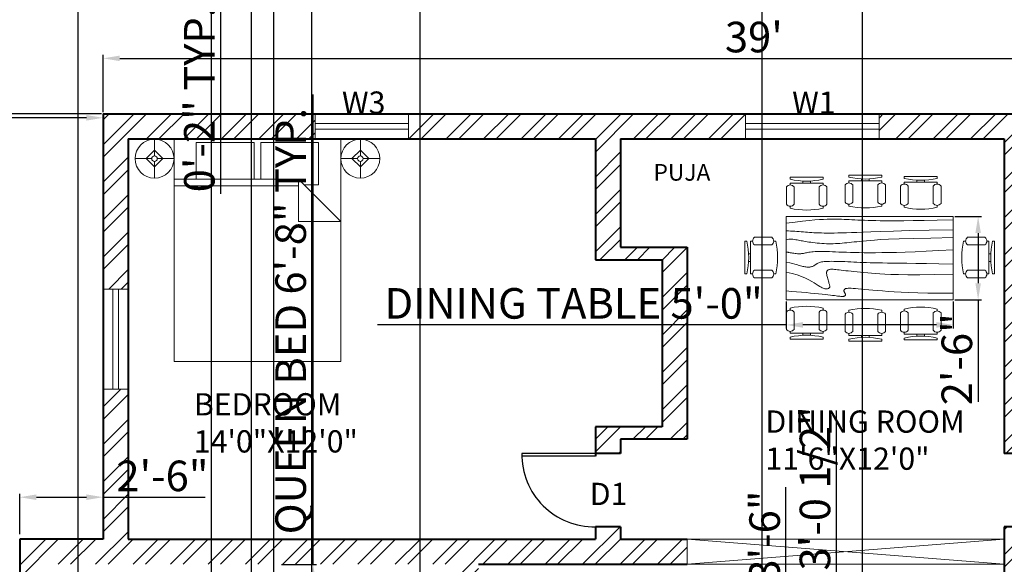
# Model space of a CAD drawing. Units: inches. Extents: x 2069 to 3028, y 691 to 1726.
# Tile 8 of 10: x 2268 to 2622, y 1325 to 1521. Entities that reach past the tile are written whole.
import ezdxf

# ---------------------------------------------------------------- set-up
doc = ezdxf.new("R2010")
doc.units = ezdxf.units.IN
for name, color, linetype, lineweight in [('A-ANNO-DIMS', 2, 'Continuous', 18), ('A-DOOR', 3, 'Continuous', 25), ('A-FURN', 8, 'Continuous', 18), ('A-GLAZ', 4, 'Continuous', 20), ('A-WALL', 7, 'Continuous', 40)]:
    doc.layers.add(name, color=color, linetype=linetype, lineweight=lineweight)
for name, color, linetype, lineweight, true_color in [('A-ANNO-TEXT', 11, 'Continuous', 18, 0xf27172), ('A-AREA-IDEN', 11, 'Continuous', 25, 0xf27172), ('A-WALL-OPEN', 143, 'Continuous', 20, 0x7aafdf), ('A-WALL-PATT', 143, 'Continuous', 13, 0x7aafdf)]:
    doc.layers.add(name, color=color, linetype=linetype, lineweight=lineweight, true_color=true_color)
doc.styles.get("Standard").update_dxf_attribs({"font": 'arial.ttf'})
doc.dimstyles.new('ISO-25', dxfattribs={"dimtxt": 11, "dimasz": 6, "dimexe": 1.25, "dimexo": 0.625, "dimtad": 1, "dimlunit": 3, "dimtxsty": 'Standard', "dimcen": 2.5, "dimclrd": 3, "dimclre": 5, "dimclrt": 6, "dimadec": 0, "dimazin": 0, "dimtfac": 1, "dimtmove": 0, "dimatfit": 3, "dimfxl": 1, "dimarcsym": 0})

# ---------------------------------------------------------------- blocks, each defined once
blk = doc.blocks.new('Table - Rectangular Woodgrain 60 x 30 in.')
for p, q in [((0, 0), (0, -30)), ((60, 0), (0, 0)), ((60, -30), (60, 0)), ((0, -30), (60, -30))]:
    blk.add_line(p, q)
for points in [[(0, -2.4), (4.8155, -2.418), (9.0302, -2.4688), (12.709, -2.5477), (15.9167, -2.65), (18.7181, -2.7711), (21.1781, -2.9063), (23.3616, -3.0508), (25.3333, -3.2), (27.1477, -3.3495), (28.8172, -3.4958), (30.3437, -3.636), (31.7291, -3.7667), (32.9756, -3.8849), (34.0849, -3.9875), (35.059, -4.0714), (35.9, -4.1334), (36.6114, -4.1711), (37.2041, -4.1854), (37.6906, -4.1779), (38.0833, -4.15), (38.3948, -4.1034), (38.6375, -4.0396), (38.8239, -3.9602), (38.9666, -3.8667), (39.0764, -3.7608), (39.1573, -3.6448), (39.2116, -3.521), (39.2416, -3.3917), (39.2498, -3.2593), (39.2385, -3.1261), (39.21, -2.9944), (39.1666, -2.8667), (39.111, -2.7447), (39.0468, -2.6281), (38.978, -2.5163), (38.9083, -2.4083), (38.8418, -2.3035), (38.7823, -2.201), (38.7337, -2.1001), (38.7, -2), (38.6844, -1.9003), (38.6875, -1.8021), (38.7094, -1.707), (38.75, -1.6167), (38.8094, -1.5326), (38.8875, -1.4563), (38.9844, -1.3893), (39.1, -1.3333), (39.2351, -1.2896), (39.3937, -1.2583), (39.5804, -1.2396), (39.8, -1.2333), (40.057, -1.2396), (40.3562, -1.2583), (40.7023, -1.2896), (41.1, -1.3333), (41.5547, -1.3895), (42.0755, -1.4573), (42.6721, -1.5361), (43.3542, -1.625), (44.1316, -1.7233), (45.014, -1.8302), (46.0114, -1.9449), (47.1333, -2.0667), (48.3862, -2.1947), (49.7625, -2.3281), (51.2513, -2.4663), (52.8416, -2.6083), (54.5226, -2.7535), (56.2833, -2.9011), (58.1127, -3.0501), (60, -3.2)], [(0, -9.2), (6.5759, -9.0858), (11.9385, -9.0365), (16.2527, -9.0418), (19.6833, -9.0917), (22.3952, -9.1759), (24.5531, -9.2844), (26.322, -9.4069), (27.8666, -9.5333), (29.3241, -9.6553), (30.7203, -9.7719), (32.0532, -9.8837), (33.3208, -9.9917), (34.5213, -10.0965), (35.6526, -10.199), (36.7128, -10.2999), (37.7, -10.4), (38.6129, -10.4996), (39.4531, -10.5969), (40.223, -10.6895), (40.925, -10.775), (41.5613, -10.8512), (42.1344, -10.9156), (42.6465, -10.966), (43.1, -11), (43.4976, -11.0158), (43.8437, -11.0136), (44.143, -10.9942), (44.4, -10.9583), (44.6195, -10.9069), (44.8062, -10.8406), (44.9648, -10.7603), (45.1, -10.6667), (45.2155, -10.5598), (45.3114, -10.4365), (45.3871, -10.2929), (45.4416, -10.125), (45.4743, -9.929), (45.4844, -9.7011), (45.4709, -9.4371), (45.4333, -9.1333), (45.3716, -8.7883), (45.2896, -8.4104), (45.1919, -8.0107), (45.0833, -7.6), (44.9685, -7.1893), (44.8521, -6.7896), (44.7388, -6.4117), (44.6333, -6.0667), (44.54, -5.7628), (44.4614, -5.4979), (44.4001, -5.2675), (44.3583, -5.0667), (44.3384, -4.8909), (44.3427, -4.7354), (44.3736, -4.5956), (44.4333, -4.4667), (44.5236, -4.3453), (44.6427, -4.2333), (44.7884, -4.1339), (44.9583, -4.05), (45.1501, -3.9849), (45.3614, -3.9417), (45.59, -3.9234), (45.8333, -3.9333), (46.0915, -3.9749), (46.3734, -4.0531), (46.6906, -4.1736), (47.0542, -4.3417), (47.4756, -4.5629), (47.9661, -4.8427), (48.5372, -5.1866), (49.2, -5.6), (49.9676, -6.0844), (50.8594, -6.625), (51.8965, -7.2031), (53.1, -7.8), (54.491, -8.3969), (56.0906, -8.975), (57.9199, -9.5156), (60, -10)], [(0, -12.8), (5.1847, -12.9322), (9.6213, -13.0323), (13.3963, -13.1059), (16.5958, -13.1583), (19.3063, -13.1952), (21.614, -13.2219), (23.6054, -13.2439), (25.3666, -13.2667), (26.9728, -13.2947), (28.4531, -13.3281), (29.8256, -13.3663), (31.1083, -13.4083), (32.3191, -13.4535), (33.476, -13.501), (34.597, -13.5501), (35.7, -13.6), (36.7984, -13.6497), (37.8875, -13.6979), (38.9578, -13.743), (40, -13.7833), (41.0047, -13.8174), (41.9625, -13.8438), (42.864, -13.8607), (43.7, -13.8667), (44.4631, -13.8604), (45.1552, -13.8417), (45.7801, -13.8104), (46.3416, -13.7667), (46.8439, -13.7104), (47.2906, -13.6417), (47.6858, -13.5604), (48.0333, -13.4667), (48.3375, -13.3608), (48.6042, -13.2448), (48.8396, -13.121), (49.05, -12.9917), (49.2417, -12.8593), (49.4208, -12.7261), (49.5937, -12.5944), (49.7667, -12.4667), (49.9452, -12.3451), (50.1323, -12.2313), (50.3303, -12.1268), (50.5416, -12.0333), (50.7686, -11.9524), (51.0135, -11.8854), (51.2788, -11.8341), (51.5666, -11.8), (51.8785, -11.7843), (52.2116, -11.7865), (52.562, -11.8059), (52.926, -11.8417), (53.2998, -11.8931), (53.6795, -11.9594), (54.0614, -12.0397), (54.4416, -12.1333), (54.8223, -12.2401), (55.2293, -12.3625), (55.6942, -12.5037), (56.2489, -12.6667), (56.9251, -12.8547), (57.7545, -13.0708), (58.7689, -13.3182), (60, -13.6)], [(0, -18), (5.124, -17.7273), (9.6609, -17.5057), (13.6705, -17.3303), (17.2125, -17.1958), (20.3467, -17.0973), (23.1328, -17.0297), (25.6307, -16.9878), (27.9, -16.9667), (29.9928, -16.9617), (31.9302, -16.9703), (33.7254, -16.9907), (35.3917, -17.0208), (36.9423, -17.0588), (38.3906, -17.1026), (39.7499, -17.1503), (41.0333, -17.2), (42.2519, -17.2496), (43.4073, -17.2969), (44.4986, -17.3395), (45.525, -17.375), (46.4858, -17.4012), (47.3802, -17.4156), (48.2074, -17.416), (48.9667, -17.4), (49.6583, -17.3662), (50.2872, -17.3167), (50.8595, -17.2547), (51.3812, -17.1833), (51.8584, -17.1057), (52.2971, -17.025), (52.7034, -16.9443), (53.0833, -16.8667), (53.443, -16.7951), (53.789, -16.7313), (54.128, -16.6768), (54.4666, -16.6334), (54.8115, -16.6024), (55.1693, -16.5854), (55.5465, -16.5841), (55.95, -16.6), (56.3828, -16.6337), (56.8346, -16.6823), (57.2915, -16.7418), (57.7396, -16.8084), (58.165, -16.878), (58.5539, -16.9469), (58.8924, -17.0111), (59.1666, -17.0667), (59.3679, -17.1107), (59.5078, -17.1438), (59.6032, -17.1675), (59.6708, -17.1833), (59.7275, -17.193), (59.7901, -17.1979), (59.8753, -17.1998), (60, -17.2)], [(0, -22.4), (8.0098, -22.2501), (14.4094, -22.1011), (19.4168, -21.9535), (23.25, -21.8083), (26.1269, -21.6663), (28.2656, -21.5281), (29.884, -21.3947), (31.2, -21.2667), (32.3967, -21.1448), (33.5172, -21.0292), (34.5697, -20.9198), (35.5625, -20.8167), (36.5037, -20.7198), (37.4015, -20.6292), (38.2642, -20.5448), (39.1, -20.4667), (39.9164, -20.3951), (40.7187, -20.3313), (41.5117, -20.2768), (42.3, -20.2333), (43.0883, -20.2024), (43.8812, -20.1854), (44.6836, -20.1841), (45.5, -20.2), (46.3328, -20.234), (47.1747, -20.2844), (48.0163, -20.3488), (48.8479, -20.425), (49.66, -20.5106), (50.4429, -20.6031), (51.1872, -20.7004), (51.8833, -20.8), (52.5246, -20.8999), (53.1166, -20.9995), (53.6681, -21.0983), (54.1875, -21.1958), (54.6834, -21.2919), (55.1646, -21.3859), (55.6394, -21.4777), (56.1167, -21.5667), (56.6028, -21.6515), (57.0961, -21.7266), (57.5929, -21.7852), (58.0896, -21.8208), (58.5823, -21.8268), (59.0674, -21.7964), (59.5412, -21.723), (60, -21.6)], [(0, -25.2), (8.6355, -25.0504), (15.7026, -24.9031), (21.4049, -24.7606), (25.9458, -24.625), (29.529, -24.4988), (32.3578, -24.3844), (34.6359, -24.284), (36.5667, -24.2), (38.3213, -24.1341), (39.9417, -24.0854), (41.437, -24.0523), (42.8167, -24.0333), (44.0901, -24.0268), (45.2667, -24.0313), (46.3557, -24.0451), (47.3667, -24.0667), (48.309, -24.0947), (49.1928, -24.1287), (50.0284, -24.168), (50.826, -24.2125), (51.5959, -24.2617), (52.3483, -24.3151), (53.0935, -24.3725), (53.8417, -24.4334), (54.6009, -24.497), (55.3699, -24.561), (56.1454, -24.6226), (56.9239, -24.6792), (57.7021, -24.7279), (58.4764, -24.7662), (59.2435, -24.7911), (60, -24.8)], [(0, -28.8), (5.6867, -28.6681), (10.45, -28.5698), (14.407, -28.5012), (17.675, -28.4584), (20.3711, -28.4374), (22.6125, -28.4344), (24.5164, -28.4455), (26.2, -28.4667), (27.762, -28.4947), (29.2276, -28.5281), (30.6033, -28.5663), (31.8958, -28.6084), (33.1118, -28.6535), (34.2578, -28.7011), (35.3405, -28.7501), (36.3666, -28.8), (37.3443, -28.8497), (38.288, -28.8974), (39.2137, -28.9412), (40.1375, -28.9792), (41.0753, -29.0093), (42.0432, -29.0297), (43.0572, -29.0384), (44.1333, -29.0333), (45.2936, -29.0114), (46.5843, -28.9641), (48.0579, -28.8816), (49.7666, -28.7542), (51.7629, -28.5721), (54.0989, -28.3255), (56.8272, -28.0048), (60, -27.6)]]:
    blk.add_lwpolyline(points)
blk = doc.blocks.new('Bed - Queen')
for p, q in [((0, -80.00003), (0, 0)), ((0, 0), (59.99999, 0)), ((59.99999, 0), (59.99999, -80.00003)), ((7.99999, -1.2), (28.79998, -1.2)), ((7.99999, -14.4), (7.99999, -1.2)), ((28.79998, -1.2), (28.79998, -14.4)), ((31.19999, -1.2), (51.99999, -1.2)), ((31.19999, -14.4), (31.19999, -1.2)), ((51.99999, -1.2), (51.99999, -16.4)), ((0, -14.4), (44.8, -14.4)), ((44.8, -16.8), (0, -16.8)), ((59.99999, -29.6), (44.8, -14.4)), ((44.8, -14.4), (44.8, -29.6)), ((51.99999, -16.4), (46.79936, -16.4)), ((44.8, -29.6), (59.99999, -29.6)), ((59.99999, -80.00003), (0, -80.00003))]:
    blk.add_line(p, q)
blk = doc.blocks.new('Lamp - Table')
for p, q in [((0, 7), (0, 1)), ((-1, 0), (-7, 0)), ((0, 3), (-3, 0)), ((-3, 0), (0, -3)), ((3, 0), (0, 3)), ((0, -3), (3, 0)), ((1, 0), (7, 0)), ((0, -1), (0, -7))]:
    blk.add_line(p, q)
for radius in [7, 1]:
    blk.add_circle((0, 0), radius)
blk = doc.blocks.new('Chair - Desk')
for p, q in [((-8.5, 0), (-8.5, -1)), ((-8.5, 0), (8.5, 0)), ((8.5, 0), (8.5, -1)), ((-10.5, -5), (-10.5, -14)), ((-8.5, -3), (-8.5, -4)), ((-8.5, -3), (8.5, -3)), ((-6.5, -14), (-6.5, -5)), ((-2, -3), (-2, -1.9355)), ((2, -1.9576), (2, -3)), ((6.5, -5), (6.5, -14)), ((8.5, -3), (8.5, -4)), ((10.5, -14), (10.5, -5)), ((-8.5, -15), (-8.5, -16)), ((8.5, -15), (8.5, -16))]:
    blk.add_line(p, q)
for centre, radius, start, end in [((-8.5, -6.5), 2.5, 36.8699, 143.1301), ((0, 34.625), 36.625, 256.5803, 283.4197), ((8.5, -6.5), 2.5, 36.8699, 143.1301), ((-8.5, -12.5), 2.5, 216.8699, 323.1301), ((8.5, -12.5), 2.5, 216.8699, 323.1301), ((0, 19.625), 36.625, 256.5803, 283.4197)]:
    blk.add_arc(centre, radius, start, end)
blk = doc.blocks.new('*D23')
at = {"layer": 'A-ANNO-DIMS', "color": 0, "lineweight": -2, "transparency": 16777216}
for p, q in [((2297.95, 1488.01), (2297.95, 1508.59)), ((2765.95, 1488.01), (2765.95, 1508.59)), ((2303.95, 1507.34), (2759.95, 1507.34))]:
    blk.add_line(p, q, dxfattribs=at)
at = {"layer": 'A-ANNO-DIMS', "color": 0, "transparency": 16777216}
for points in [[(2303.95, 1508.34), (2303.95, 1506.34), (2297.95, 1507.34)], [(2759.95, 1508.34), (2759.95, 1506.34), (2765.95, 1507.34)]]:
    blk.add_solid(points, dxfattribs=at)
at = {"layer": 'Defpoints', "color": 0, "transparency": 16777216}
for p in [(2765.95, 1507.34), (2297.95, 1487.39), (2765.95, 1487.39)]:
    blk.add_point(p, dxfattribs=at)
at = {"layer": 'A-ANNO-DIMS', "color": 0, "transparency": 16777216, "insert": (2531.95, 1513.58), "char_height": 11, "attachment_point": 5}
blk.add_mtext("39'", dxfattribs=at)
blk = doc.blocks.new('*D35')
at = {"layer": 'A-ANNO-DIMS', "color": 0, "lineweight": -2, "transparency": 16777216}
for p, q in [((2267.95, 1336.26), (2267.95, 1350.77)), ((2273.95, 1349.52), (2291.95, 1349.52)), ((2297.95, 1336.26), (2297.95, 1350.77)), ((2297.95, 1349.52), (2334.63, 1349.52))]:
    blk.add_line(p, q, dxfattribs=at)
at = {"layer": 'A-ANNO-DIMS', "color": 0, "transparency": 16777216}
for points in [[(2273.95, 1350.52), (2273.95, 1348.52), (2267.95, 1349.52)], [(2291.95, 1350.52), (2291.95, 1348.52), (2297.95, 1349.52)]]:
    blk.add_solid(points, dxfattribs=at)
at = {"layer": 'Defpoints', "color": 0, "transparency": 16777216}
for p in [(2297.95, 1349.52), (2267.95, 1335.64), (2297.95, 1335.64)]:
    blk.add_point(p, dxfattribs=at)
at = {"layer": 'A-ANNO-DIMS', "color": 0, "transparency": 16777216, "insert": (2319.29, 1355.76), "char_height": 11, "attachment_point": 5}
blk.add_mtext('2\'-6"', dxfattribs=at)
blk = doc.blocks.new('*D36')
at = {"layer": 'A-ANNO-DIMS', "color": 0, "lineweight": -2, "transparency": 16777216}
for p, q in [((2150.95, 1486.76), (2150.95, 1484.71)), ((2291.95, 1485.96), (2156.95, 1485.96)), ((2297.95, 1486.76), (2297.95, 1484.71))]:
    blk.add_line(p, q, dxfattribs=at)
at = {"layer": 'A-ANNO-DIMS', "color": 0, "transparency": 16777216}
for points in [[(2156.95, 1486.96), (2156.95, 1484.96), (2150.95, 1485.96)], [(2291.95, 1486.96), (2291.95, 1484.96), (2297.95, 1485.96)]]:
    blk.add_solid(points, dxfattribs=at)
at = {"layer": 'Defpoints', "color": 0, "transparency": 16777216}
for p in [(2150.95, 1487.39), (2297.95, 1487.39), (2150.95, 1485.96)]:
    blk.add_point(p, dxfattribs=at)
at = {"layer": 'A-ANNO-DIMS', "color": 0, "transparency": 16777216, "insert": (2224.45, 1492.21), "char_height": 11, "attachment_point": 5}
blk.add_mtext('12\'-3"', dxfattribs=at)
blk = doc.blocks.new('DOOR-SWING-26_4IN')
for p, q in [((0, 0), (-26.4, 0)), ((0, -1), (-26.4, -1))]:
    blk.add_line(p, q)
blk.add_arc((-0.5, -0.5), 25.9, 178.894, 271.106)
blk = doc.blocks.new('WINDOW-36IN')
for p, q in [((0, 0), (9, 0)), ((3.5, 0), (3.5, -36)), ((5.5, 0), (5.5, -36)), ((0, -36), (9, -36))]:
    blk.add_line(p, q)
blk = doc.blocks.new('WINDOW-SASH-48IN')
for p, q in [((0, 0), (48, 0)), ((0, -2), (48, -2))]:
    blk.add_line(p, q)
blk = doc.blocks.new('WINDOW-SASH-33_6IN')
for p, q in [((0, 0), (33.6, 0)), ((0, -2), (33.6, -2))]:
    blk.add_line(p, q)
blk = doc.blocks.new('*D54')
at = {"layer": 'A-ANNO-DIMS', "color": 3, "lineweight": -2, "transparency": 16777216}
for p, q in [((2373.46, 1325.32), (2373.46, 1494.38)), ((2373.46, 1251.32), (2373.46, 1319.32))]:
    blk.add_line(p, q, dxfattribs=at)
at = {"layer": 'A-ANNO-DIMS', "color": 5, "lineweight": -2, "transparency": 16777216}
for p, q in [((2362.09, 1325.32), (2374.71, 1325.32)), ((2362.09, 1245.32), (2374.71, 1245.32))]:
    blk.add_line(p, q, dxfattribs=at)
at = {"layer": 'A-ANNO-DIMS', "color": 3, "transparency": 16777216}
for points in [[(2372.46, 1319.32), (2374.46, 1319.32), (2373.46, 1325.32)], [(2372.46, 1251.32), (2374.46, 1251.32), (2373.46, 1245.32)]]:
    blk.add_solid(points, dxfattribs=at)
at = {"layer": 'Defpoints', "color": 0, "transparency": 16777216}
for p in [(2361.46, 1325.32), (2373.46, 1325.32), (2361.46, 1245.32)]:
    blk.add_point(p, dxfattribs=at)
at = {"layer": 'A-ANNO-DIMS', "color": 6, "transparency": 16777216, "insert": (2366.81, 1412.85), "char_height": 11, "attachment_point": 5, "rotation": 90}
blk.add_mtext('QUEEN BED 6\'-8" TYP.', dxfattribs=at)
blk = doc.blocks.new('*D60')
at = {"layer": 'A-ANNO-DIMS', "color": 3, "lineweight": -2, "transparency": 16777216}
for p, q in [((2345.25, 1545.93), (2217.55, 1545.93)), ((2372.85, 1545.93), (2351.25, 1545.93))]:
    blk.add_line(p, q, dxfattribs=at)
at = {"layer": 'A-ANNO-DIMS', "color": 5, "lineweight": -2, "transparency": 16777216}
for p, q in [((2345.25, 1541.51), (2345.25, 1547.18)), ((2378.85, 1541.51), (2378.85, 1547.18))]:
    blk.add_line(p, q, dxfattribs=at)
at = {"layer": 'A-ANNO-DIMS', "color": 3, "transparency": 16777216}
for points in [[(2351.25, 1546.93), (2351.25, 1544.93), (2345.25, 1545.93)], [(2372.85, 1546.93), (2372.85, 1544.93), (2378.85, 1545.93)]]:
    blk.add_solid(points, dxfattribs=at)
at = {"layer": 'Defpoints', "color": 0, "transparency": 16777216}
for p in [(2345.25, 1545.93), (2345.25, 1540.89), (2378.85, 1540.89)]:
    blk.add_point(p, dxfattribs=at)
at = {"layer": 'A-ANNO-DIMS', "color": 6, "transparency": 16777216, "insert": (2278.4, 1552.24), "char_height": 11, "attachment_point": 5}
blk.add_mtext('W3 2\'-9 1/2" TYP.', dxfattribs=at)
blk = doc.blocks.new('*D61')
at = {"layer": 'A-ANNO-DIMS', "color": 3, "lineweight": -2, "transparency": 16777216}
for p, q in [((2340.21, 1546.89), (2340.21, 1552.89)), ((2340.21, 1540.89), (2340.21, 1538.89)), ((2340.21, 1532.89), (2340.21, 1458.59))]:
    blk.add_line(p, q, dxfattribs=at)
at = {"layer": 'A-ANNO-DIMS', "color": 5, "lineweight": -2, "transparency": 16777216}
for p, q in [((2344.62, 1540.89), (2338.96, 1540.89)), ((2344.62, 1538.89), (2338.96, 1538.89))]:
    blk.add_line(p, q, dxfattribs=at)
at = {"layer": 'A-ANNO-DIMS', "color": 3, "transparency": 16777216}
for points in [[(2339.21, 1546.89), (2341.21, 1546.89), (2340.21, 1540.89)], [(2339.21, 1532.89), (2341.21, 1532.89), (2340.21, 1538.89)]]:
    blk.add_solid(points, dxfattribs=at)
at = {"layer": 'Defpoints', "color": 0, "transparency": 16777216}
for p in [(2345.25, 1540.89), (2340.21, 1538.89), (2345.25, 1538.89)]:
    blk.add_point(p, dxfattribs=at)
at = {"layer": 'A-ANNO-DIMS', "color": 6, "transparency": 16777216, "insert": (2333.97, 1492.74), "char_height": 11, "attachment_point": 5, "rotation": 90}
blk.add_mtext('0\'-2" TYP.', dxfattribs=at)
blk = doc.blocks.new('*D68')
at = {"layer": 'A-ANNO-DIMS', "color": 3, "lineweight": -2, "transparency": 16777216}
for p, q in [((2543.48, 1263.36), (2543.48, 1353.08)), ((2543.48, 1227.27), (2543.48, 1257.36))]:
    blk.add_line(p, q, dxfattribs=at)
at = {"layer": 'A-ANNO-DIMS', "color": 5, "lineweight": -2, "transparency": 16777216}
for p, q in [((2537.79, 1263.36), (2544.73, 1263.36)), ((2537.79, 1221.27), (2544.73, 1221.27))]:
    blk.add_line(p, q, dxfattribs=at)
at = {"layer": 'A-ANNO-DIMS', "color": 3, "transparency": 16777216}
for points in [[(2542.48, 1257.36), (2544.48, 1257.36), (2543.48, 1263.36)], [(2542.48, 1227.27), (2544.48, 1227.27), (2543.48, 1221.27)]]:
    blk.add_solid(points, dxfattribs=at)
at = {"layer": 'Defpoints', "color": 0, "transparency": 16777216}
for p in [(2537.16, 1263.36), (2543.48, 1263.36), (2537.16, 1221.27)]:
    blk.add_point(p, dxfattribs=at)
at = {"layer": 'A-ANNO-DIMS', "color": 6, "transparency": 16777216, "insert": (2537.23, 1311.22), "char_height": 11, "attachment_point": 5, "rotation": 90}
blk.add_mtext('TABLE 3\'-6"', dxfattribs=at)
blk = doc.blocks.new('*D78')
at = {"layer": 'A-ANNO-DIMS', "color": 5, "lineweight": -2, "transparency": 16777216}
for p, q in [((2543.59, 1419.86), (2543.59, 1410.23)), ((2603.59, 1419.86), (2603.59, 1410.23))]:
    blk.add_line(p, q, dxfattribs=at)
at = {"layer": 'A-ANNO-DIMS', "color": 3, "lineweight": -2, "transparency": 16777216}
for p, q in [((2543.59, 1411.48), (2396.64, 1411.48)), ((2597.59, 1411.48), (2549.59, 1411.48))]:
    blk.add_line(p, q, dxfattribs=at)
at = {"layer": 'A-ANNO-DIMS', "color": 3, "transparency": 16777216}
for points in [[(2549.59, 1412.48), (2549.59, 1410.48), (2543.59, 1411.48)], [(2597.59, 1412.48), (2597.59, 1410.48), (2603.59, 1411.48)]]:
    blk.add_solid(points, dxfattribs=at)
at = {"layer": 'Defpoints', "color": 0, "transparency": 16777216}
for p in [(2543.59, 1420.48), (2603.59, 1420.48), (2543.59, 1411.48)]:
    blk.add_point(p, dxfattribs=at)
at = {"layer": 'A-ANNO-DIMS', "color": 6, "transparency": 16777216, "insert": (2467.12, 1417.8), "char_height": 11, "attachment_point": 5}
blk.add_mtext('DINING TABLE 5\'-0"', dxfattribs=at)
blk = doc.blocks.new('*D79')
at = {"layer": 'A-ANNO-DIMS', "color": 5, "lineweight": -2, "transparency": 16777216}
for p, q in [((2604.21, 1450.48), (2613.84, 1450.48)), ((2604.21, 1420.48), (2613.84, 1420.48))]:
    blk.add_line(p, q, dxfattribs=at)
at = {"layer": 'A-ANNO-DIMS', "color": 3, "lineweight": -2, "transparency": 16777216}
for p, q in [((2612.59, 1444.48), (2612.59, 1426.48)), ((2612.59, 1420.48), (2612.59, 1383.8))]:
    blk.add_line(p, q, dxfattribs=at)
at = {"layer": 'A-ANNO-DIMS', "color": 3, "transparency": 16777216}
for points in [[(2611.59, 1444.48), (2613.59, 1444.48), (2612.59, 1450.48)], [(2611.59, 1426.48), (2613.59, 1426.48), (2612.59, 1420.48)]]:
    blk.add_solid(points, dxfattribs=at)
at = {"layer": 'Defpoints', "color": 0, "transparency": 16777216}
for p in [(2603.59, 1450.48), (2603.59, 1420.48), (2612.59, 1420.48)]:
    blk.add_point(p, dxfattribs=at)
at = {"layer": 'A-ANNO-DIMS', "color": 6, "transparency": 16777216, "insert": (2606.35, 1399.14), "char_height": 11, "attachment_point": 5, "rotation": 90}
blk.add_mtext('2\'-6"', dxfattribs=at)
blk = doc.blocks.new('*D81')
at = {"layer": 'A-ANNO-DIMS', "color": 3, "lineweight": -2, "transparency": 16777216}
for p, q in [((2561.66, 1318.63), (2561.66, 1380.74)), ((2561.66, 1287.96), (2561.66, 1312.63))]:
    blk.add_line(p, q, dxfattribs=at)
at = {"layer": 'A-ANNO-DIMS', "color": 5, "lineweight": -2, "transparency": 16777216}
for p, q in [((2553.28, 1318.63), (2562.91, 1318.63)), ((2553.28, 1281.96), (2562.91, 1281.96))]:
    blk.add_line(p, q, dxfattribs=at)
at = {"layer": 'A-ANNO-DIMS', "color": 3, "transparency": 16777216}
for points in [[(2560.66, 1312.63), (2562.66, 1312.63), (2561.66, 1318.63)], [(2560.66, 1287.96), (2562.66, 1287.96), (2561.66, 1281.96)]]:
    blk.add_solid(points, dxfattribs=at)
at = {"layer": 'Defpoints', "color": 0, "transparency": 16777216}
for p in [(2552.66, 1318.63), (2561.66, 1318.63), (2552.66, 1281.96)]:
    blk.add_point(p, dxfattribs=at)
at = {"layer": 'A-ANNO-DIMS', "color": 6, "transparency": 16777216, "insert": (2555.34, 1352.69), "char_height": 11, "attachment_point": 5, "rotation": 90}
blk.add_mtext('3\'-0 1/2"', dxfattribs=at)
blk = doc.blocks.new('*D87')
at = {"layer": 'A-ANNO-DIMS', "color": 5, "lineweight": -2, "transparency": 16777216}
for p, q in [((2297.33, 1487.39), (2090.2, 1487.39)), ((2297.33, 903.89), (2090.2, 903.89))]:
    blk.add_line(p, q, dxfattribs=at)
at = {"layer": 'A-ANNO-DIMS', "color": 3, "lineweight": -2, "transparency": 16777216}
blk.add_line((2091.45, 909.89), (2091.45, 1481.39), dxfattribs=at)
at = {"layer": 'A-ANNO-DIMS', "color": 3, "transparency": 16777216}
for points in [[(2090.45, 1481.39), (2092.45, 1481.39), (2091.45, 1487.39)], [(2090.45, 909.89), (2092.45, 909.89), (2091.45, 903.89)]]:
    blk.add_solid(points, dxfattribs=at)
at = {"layer": 'Defpoints', "color": 0, "transparency": 16777216}
for p in [(2091.45, 1487.39), (2297.95, 1487.39), (2297.95, 903.89)]:
    blk.add_point(p, dxfattribs=at)
at = {"layer": 'A-ANNO-DIMS', "color": 6, "transparency": 16777216, "insert": (2085.14, 1195.64), "char_height": 11, "attachment_point": 5, "rotation": 90}
blk.add_mtext('48\'-7 1/2"', dxfattribs=at)
blk = doc.blocks.new('*D88')
at = {"layer": 'A-ANNO-DIMS', "color": 5, "lineweight": -2, "transparency": 16777216}
for p, q in [((2288.92, 738.01), (2288.92, 1704.14)), ((2336.92, 738.01), (2336.92, 1704.14))]:
    blk.add_line(p, q, dxfattribs=at)
at = {"layer": 'A-ANNO-DIMS', "color": 3, "lineweight": -2, "transparency": 16777216}
blk.add_line((2294.92, 1702.89), (2330.92, 1702.89), dxfattribs=at)
at = {"layer": 'A-ANNO-DIMS', "color": 3, "transparency": 16777216}
for points in [[(2294.92, 1703.89), (2294.92, 1701.89), (2288.92, 1702.89)], [(2330.92, 1703.89), (2330.92, 1701.89), (2336.92, 1702.89)]]:
    blk.add_solid(points, dxfattribs=at)
at = {"layer": 'Defpoints', "color": 0, "transparency": 16777216}
for p in [(2336.92, 1702.89), (2288.92, 737.39), (2336.92, 737.39)]:
    blk.add_point(p, dxfattribs=at)
at = {"layer": 'A-ANNO-DIMS', "color": 6, "transparency": 16777216, "insert": (2312.92, 1709.13), "char_height": 11, "attachment_point": 5}
blk.add_mtext('4\'-0"', dxfattribs=at)
blk = doc.blocks.new('*D89')
at = {"layer": 'A-ANNO-DIMS', "color": 5, "lineweight": -2, "transparency": 16777216}
for p, q in [((2336.92, 747.01), (2336.92, 1704.14)), ((2711.95, 747.01), (2711.95, 1704.14))]:
    blk.add_line(p, q, dxfattribs=at)
at = {"layer": 'A-ANNO-DIMS', "color": 3, "lineweight": -2, "transparency": 16777216}
blk.add_line((2342.92, 1702.89), (2705.95, 1702.89), dxfattribs=at)
at = {"layer": 'A-ANNO-DIMS', "color": 3, "transparency": 16777216}
for points in [[(2342.92, 1703.89), (2342.92, 1701.89), (2336.92, 1702.89)], [(2705.95, 1703.89), (2705.95, 1701.89), (2711.95, 1702.89)]]:
    blk.add_solid(points, dxfattribs=at)
at = {"layer": 'Defpoints', "color": 0, "transparency": 16777216}
for p in [(2711.95, 1702.89), (2336.92, 746.39), (2711.95, 746.39)]:
    blk.add_point(p, dxfattribs=at)
at = {"layer": 'A-ANNO-DIMS', "color": 6, "transparency": 16777216, "insert": (2524.44, 1709.13), "char_height": 11, "attachment_point": 5}
blk.add_mtext('31\'-3"', dxfattribs=at)
blk = doc.blocks.new('*D91')
at = {"layer": 'A-ANNO-DIMS', "color": 5, "lineweight": -2, "transparency": 16777216}
for p, q in [((2289.83, 1535.39), (2090.2, 1535.39)), ((2297.33, 1487.39), (2090.2, 1487.39))]:
    blk.add_line(p, q, dxfattribs=at)
at = {"layer": 'A-ANNO-DIMS', "color": 3, "lineweight": -2, "transparency": 16777216}
blk.add_line((2091.45, 1529.39), (2091.45, 1493.39), dxfattribs=at)
at = {"layer": 'A-ANNO-DIMS', "color": 3, "transparency": 16777216}
for points in [[(2090.45, 1529.39), (2092.45, 1529.39), (2091.45, 1535.39)], [(2090.45, 1493.39), (2092.45, 1493.39), (2091.45, 1487.39)]]:
    blk.add_solid(points, dxfattribs=at)
at = {"layer": 'Defpoints', "color": 0, "transparency": 16777216}
for p in [(2290.45, 1535.39), (2091.45, 1487.39), (2297.95, 1487.39)]:
    blk.add_point(p, dxfattribs=at)
at = {"layer": 'A-ANNO-DIMS', "color": 6, "transparency": 16777216, "insert": (2085.21, 1511.39), "char_height": 11, "attachment_point": 5, "rotation": 90}
blk.add_mtext('4\'-0"', dxfattribs=at)
blk = doc.blocks.new('*D92')
at = {"layer": 'A-ANNO-DIMS', "color": 5, "lineweight": -2, "transparency": 16777216}
for p, q in [((2359.37, 992.45), (2359.37, 1704.14)), ((2411.94, 992.45), (2411.94, 1704.14))]:
    blk.add_line(p, q, dxfattribs=at)
at = {"layer": 'A-ANNO-DIMS', "color": 3, "lineweight": -2, "transparency": 16777216}
for p, q in [((2365.37, 1702.89), (2405.94, 1702.89)), ((2411.94, 1702.89), (2474.5, 1702.89))]:
    blk.add_line(p, q, dxfattribs=at)
at = {"layer": 'A-ANNO-DIMS', "color": 3, "transparency": 16777216}
for points in [[(2365.37, 1703.89), (2365.37, 1701.89), (2359.37, 1702.89)], [(2405.94, 1703.89), (2405.94, 1701.89), (2411.94, 1702.89)]]:
    blk.add_solid(points, dxfattribs=at)
at = {"layer": 'Defpoints', "color": 0, "transparency": 16777216}
for p in [(2411.94, 1702.89), (2359.37, 991.83), (2411.94, 991.83)]:
    blk.add_point(p, dxfattribs=at)
at = {"layer": 'A-ANNO-DIMS', "color": 6, "transparency": 16777216, "insert": (2446.22, 1709.2), "char_height": 11, "attachment_point": 5}
blk.add_mtext('4\'-4 1/2"', dxfattribs=at)
blk = doc.blocks.new('*D95')
at = {"layer": 'A-ANNO-DIMS', "color": 5, "lineweight": -2, "transparency": 16777216}
for p, q in [((2351.35, 1134.01), (2351.35, 1704.14)), ((2372.95, 1134.01), (2372.95, 1704.14))]:
    blk.add_line(p, q, dxfattribs=at)
at = {"layer": 'A-ANNO-DIMS', "color": 3, "lineweight": -2, "transparency": 16777216}
for p, q in [((2357.35, 1702.89), (2366.95, 1702.89)), ((2372.95, 1702.89), (2434.04, 1702.89))]:
    blk.add_line(p, q, dxfattribs=at)
at = {"layer": 'A-ANNO-DIMS', "color": 3, "transparency": 16777216}
for points in [[(2357.35, 1703.89), (2357.35, 1701.89), (2351.35, 1702.89)], [(2366.95, 1703.89), (2366.95, 1701.89), (2372.95, 1702.89)]]:
    blk.add_solid(points, dxfattribs=at)
at = {"layer": 'Defpoints', "color": 0, "transparency": 16777216}
for p in [(2372.95, 1702.89), (2351.35, 1133.39), (2372.95, 1133.39)]:
    blk.add_point(p, dxfattribs=at)
at = {"layer": 'A-ANNO-DIMS', "color": 6, "transparency": 16777216, "insert": (2406.49, 1709.2), "char_height": 11, "attachment_point": 5}
blk.add_mtext('1\'-9 1/2"', dxfattribs=at)
blk = doc.blocks.new('*D96')
at = {"layer": 'A-ANNO-DIMS', "color": 5, "lineweight": -2, "transparency": 16777216}
for p, q in [((2534.95, 1066.51), (2534.95, 1704.14)), ((2570.95, 1066.51), (2570.95, 1704.14))]:
    blk.add_line(p, q, dxfattribs=at)
at = {"layer": 'A-ANNO-DIMS', "color": 3, "lineweight": -2, "transparency": 16777216}
blk.add_line((2540.95, 1702.89), (2564.95, 1702.89), dxfattribs=at)
at = {"layer": 'A-ANNO-DIMS', "color": 3, "transparency": 16777216}
for points in [[(2540.95, 1703.89), (2540.95, 1701.89), (2534.95, 1702.89)], [(2564.95, 1703.89), (2564.95, 1701.89), (2570.95, 1702.89)]]:
    blk.add_solid(points, dxfattribs=at)
at = {"layer": 'Defpoints', "color": 0, "transparency": 16777216}
for p in [(2570.95, 1702.89), (2534.95, 1065.89), (2570.95, 1065.89)]:
    blk.add_point(p, dxfattribs=at)
at = {"layer": 'A-ANNO-DIMS', "color": 6, "transparency": 16777216, "insert": (2552.95, 1709.13), "char_height": 11, "attachment_point": 5}
blk.add_mtext('3\'-0"', dxfattribs=at)

msp = doc.modelspace()

# ---------------------------------------------------------------- hatches: boundary and pattern name
at = {"layer": 'A-WALL-PATT'}
h = msp.add_hatch(dxfattribs=at)
h.set_pattern_fill('ANSI32', color=256)
h.paths.add_polyline_path([(2675.951, 1487.387), (2576.951, 1487.387), (2576.951, 1478.387), (2621.951, 1478.387), (2621.951, 1365.287), (2630.951, 1365.287), (2630.951, 1478.387), (2675.951, 1478.387)])
h.paths.add_polyline_path([(2765.951, 1487.387), (2711.951, 1487.387), (2711.951, 1478.387), (2756.951, 1478.387), (2756.951, 1424.387), (2765.951, 1424.387)])
h.paths.add_polyline_path([(2528.951, 1487.387), (2407.751, 1487.387), (2407.751, 1478.387), (2474.951, 1478.387), (2474.951, 1434.887), (2498.951, 1434.887), (2498.951, 1374.887), (2474.951, 1374.887), (2474.951, 1365.287), (2483.951, 1365.287), (2483.951, 1370.387), (2507.951, 1370.387), (2507.951, 1439.387), (2483.951, 1439.387), (2483.951, 1478.387), (2528.951, 1478.387)])
h.paths.add_polyline_path([(2374.151, 1487.387), (2297.951, 1487.387), (2297.951, 1424.387), (2306.951, 1424.387), (2306.951, 1478.387), (2374.151, 1478.387)])
h.paths.add_polyline_path([(2507.951, 1334.387), (2483.951, 1334.387), (2483.951, 1338.887), (2474.951, 1338.887), (2474.951, 1334.387), (2306.951, 1334.387), (2306.951, 1388.387), (2297.951, 1388.387), (2297.951, 1334.387), (2267.951, 1334.387), (2267.951, 1274.387), (2276.951, 1274.387), (2276.951, 1325.387), (2297.951, 1325.387), (2423.951, 1325.387), (2423.951, 1187.387), (2419.451, 1187.387), (2419.451, 1178.387), (2432.951, 1178.387), (2432.951, 1325.387), (2507.951, 1325.387)])
h.paths.add_polyline_path([(2795.951, 1334.387), (2630.951, 1334.387), (2630.951, 1338.887), (2621.951, 1338.887), (2621.951, 1178.387), (2635.451, 1178.387), (2635.451, 1187.387), (2630.951, 1187.387), (2630.951, 1325.387), (2786.951, 1325.387), (2786.951, 1274.387), (2795.951, 1274.387)])
h.paths.add_polyline_path([(2765.951, 1388.387), (2756.951, 1388.387), (2756.951, 1334.387), (2765.951, 1334.387)])
h.paths.add_polyline_path([(2795.951, 1238.387), (2786.951, 1238.387), (2786.951, 1187.387), (2665.451, 1187.387), (2665.451, 1178.387), (2795.951, 1178.387)], flags=17)
h.paths.add_polyline_path([(2389.451, 1187.387), (2276.951, 1187.387), (2276.951, 1238.387), (2267.951, 1238.387), (2267.951, 1178.387), (2297.951, 1178.387), (2297.951, 1173.287), (2307.451, 1173.287), (2307.451, 1178.387), (2389.451, 1178.387)])
h.paths.add_polyline_path([(2377.451, 1142.387), (2306.951, 1142.387), (2306.951, 1146.887), (2297.951, 1146.887), (2297.951, 1142.387), (2297.951, 1137.887), (2306.951, 1137.887), (2372.951, 1137.887), (2372.951, 1133.387), (2377.451, 1133.387)])
h.paths.add_polyline_path([(2795.951, 1065.887), (2665.451, 1065.887), (2665.451, 1056.887), (2786.951, 1056.887), (2786.951, 1002.887), (2795.951, 1002.887), (2795.951, 1056.887)])
h.paths.add_polyline_path([(2795.951, 966.887), (2786.951, 966.887), (2786.951, 912.887), (2732.951, 912.887), (2732.951, 903.887), (2795.951, 903.887)])
h.paths.add_polyline_path([(2483.951, 917.387), (2474.951, 917.387), (2474.951, 912.887), (2414.951, 912.887), (2414.951, 903.887), (2483.951, 903.887)])
h.paths.add_polyline_path([(2366.951, 912.887), (2306.951, 912.887), (2306.951, 960.887), (2297.951, 960.887), (2297.951, 903.887), (2366.951, 903.887)])
h.paths.add_polyline_path([(2498.951, 1056.887), (2498.951, 1065.887), (2377.451, 1065.887), (2377.451, 1111.787), (2372.951, 1111.787), (2372.951, 1065.887), (2306.951, 1065.887), (2306.951, 1116.287), (2297.951, 1116.287), (2297.951, 1056.887), (2297.951, 1008.887), (2306.951, 1008.887), (2306.951, 1056.887), (2474.951, 1056.887), (2474.951, 947.387), (2483.951, 947.387), (2483.951, 1056.887)])

# ---------------------------------------------------------------- linework, layer by layer
at = {"layer": 'A-GLAZ'}
for p, q in [((2374.151, 1487.387), (2374.151, 1478.387)), ((2407.751, 1487.387), (2407.751, 1478.387)), ((2528.951, 1487.387), (2528.951, 1478.387)), ((2576.951, 1487.387), (2576.951, 1478.387))]:
    msp.add_line(p, q, dxfattribs=at)
at = {"layer": 'A-WALL'}
for p, q in [((2297.951, 1487.387), (2765.951, 1487.387)), ((2297.951, 1487.387), (2297.951, 1334.387)), ((2306.951, 1478.387), (2306.951, 1334.387)), ((2306.951, 1478.387), (2474.951, 1478.387)), ((2474.951, 1478.387), (2474.951, 1434.887)), ((2483.951, 1478.387), (2483.951, 1439.387)), ((2483.951, 1478.387), (2621.951, 1478.387)), ((2621.951, 1478.387), (2621.951, 1365.287)), ((2483.951, 1439.387), (2507.951, 1439.387)), ((2507.951, 1439.387), (2507.951, 1379.387)), ((2507.951, 1439.387), (2507.951, 1370.387)), ((2474.951, 1434.887), (2498.951, 1434.887)), ((2498.951, 1434.887), (2498.951, 1374.887)), ((2474.951, 1374.887), (2474.951, 1364.287)), ((2498.951, 1374.887), (2474.951, 1374.887)), ((2507.951, 1370.387), (2483.951, 1370.387)), ((2483.951, 1370.387), (2483.951, 1365.287)), ((2483.951, 1365.287), (2474.951, 1365.287)), ((2630.951, 1365.287), (2621.951, 1365.287)), ((2483.951, 1338.887), (2474.951, 1338.887)), ((2474.951, 1338.887), (2474.951, 1334.387)), ((2483.951, 1338.887), (2483.951, 1334.387)), ((2630.951, 1338.887), (2621.951, 1338.887)), ((2621.951, 1338.887), (2621.951, 1178.387)), ((2297.951, 1334.387), (2267.951, 1334.387)), ((2267.951, 1334.387), (2267.951, 1178.387)), ((2306.951, 1334.387), (2474.951, 1334.387)), ((2483.951, 1334.387), (2507.951, 1334.387)), ((2432.951, 1325.387), (2507.951, 1325.387))]:
    msp.add_line(p, q, dxfattribs=at)
at = {"layer": 'A-WALL-OPEN'}
for p, q in [((2507.951, 1334.387), (2507.951, 1325.387)), ((2621.951, 1334.387), (2507.951, 1325.387)), ((2507.951, 1334.387), (2621.951, 1325.387)), ((2507.951, 1334.387), (2621.951, 1334.387)), ((2507.951, 1325.387), (2621.951, 1325.387))]:
    msp.add_line(p, q, dxfattribs=at)

# ---------------------------------------------------------------- block references
at = {"layer": 'A-DOOR'}
msp.add_blockref('DOOR-SWING-26_4IN', (2474.951, 1365.287), dxfattribs=at)
at = {"layer": 'A-FURN'}
for name, p in [('Lamp - Table', (2316.441, 1471.271)), ('Bed - Queen', (2323.441, 1478.271))]:
    msp.add_blockref(name, p, dxfattribs=at)
at = {"layer": 'A-FURN', "xscale": -1}
msp.add_blockref('Lamp - Table', (2390.441, 1471.271), dxfattribs=at)
at = {"layer": 'A-FURN', "xscale": 0.6944950846218003, "yscale": 0.6944950846218003, "zscale": 0.6944950846218003}
for p in [(2550.915, 1464.576), (2572.014, 1465.334), (2591.943, 1464.888)]:
    msp.add_blockref('Chair - Desk', p, dxfattribs=at)
at = {"layer": 'A-FURN', "rotation": 180}
msp.add_blockref('Table - Rectangular Woodgrain 60 x 30 in.', (2603.59, 1420.483), dxfattribs=at)
at = {"layer": 'A-FURN', "yscale": 0.6944950846218003, "zscale": 0.6944950846218003}
for p, xscale, rotation in [((2528.689, 1435.711), 0.6944950846218003, 90), ((2618.49, 1435.711), -0.6944950846218003, 270), ((2550.915, 1406.39), -0.6944950846218003, 180), ((2572.014, 1405.633), -0.6944950846218003, 180), ((2591.943, 1406.078), -0.6944950846218003, 180)]:
    msp.add_blockref('Chair - Desk', p, dxfattribs=dict(at, xscale=xscale, rotation=rotation))
at = {"layer": 'A-GLAZ', "rotation": 180}
for name, p in [('WINDOW-SASH-33_6IN', (2407.751, 1481.887)), ('WINDOW-36IN', (2306.951, 1388.387))]:
    msp.add_blockref(name, p, dxfattribs=at)
at = {"layer": 'A-GLAZ'}
msp.add_blockref('WINDOW-SASH-48IN', (2528.951, 1483.887), dxfattribs=at)

# ---------------------------------------------------------------- texts
at = {"layer": 'A-ANNO-TEXT', "char_height": 8, "attachment_point": 1}
for s, insert in [('{\\fArial|b1|i0|c0|p34;W3}', (2383.824, 1495.419)), ('{\\fArial|b1|i0|c0|p34;W1}', (2545.711, 1495.419)), ('{\\fArial|b1|i0|c0|p34;D1}', (2472.925, 1354.696))]:
    msp.add_mtext_dynamic_manual_height_columns(s, width=34.05605, gutter_width=12.5, heights=[0], dxfattribs=dict(at, insert=insert))
at = {"layer": 'A-AREA-IDEN', "attachment_point": 1}
for s, heights, insert, char_height in [(' PUJA', [6.102], (2494.029, 1469.346), 6), ('BEDROOM\\P14\'0"X12\'0"', [0], (2330.547, 1386.931), 8), ('DINING ROOM\\P11\'6"X12\'0"', [0], (2536.103, 1380.715), 8)]:
    msp.add_mtext_dynamic_manual_height_columns(s, width=119.20948, gutter_width=12.5, heights=heights, dxfattribs=dict(at, insert=insert, char_height=char_height))

# ---------------------------------------------------------------- dimensions: what is measured, and where the dimension line sits
at = {"layer": 'A-ANNO-DIMS'}
for base, p1, p2, override, picture, middle in [((2372.951, 1702.887), (2351.351, 1133.387), (2372.951, 1133.387), {"dimdec": 1, "dimlfac": 1, "dimrnd": 0, "dimzin": 1, "dimdsep": 46, "dimlunit": 4, "dimfrac": 2}, '*D95', (2406.495, 1709.199)), ((2411.936, 1702.887), (2359.366, 991.83), (2411.936, 991.83), {"dimdec": 1, "dimlfac": 1, "dimrnd": 0, "dimzin": 1, "dimdsep": 46, "dimlunit": 4, "dimfrac": 2}, '*D92', (2446.219, 1709.199)), ((2336.919, 1702.887), (2288.919, 737.387), (2336.919, 737.387), {"dimdec": 1, "dimlfac": 1, "dimrnd": 0, "dimzin": 1, "dimdsep": 46, "dimlunit": 4, "dimfrac": 2}, '*D88', (2312.919, 1709.128)), ((2711.951, 1702.887), (2336.919, 746.387), (2711.951, 746.387), {"dimdec": 1, "dimlfac": 1, "dimrnd": 0, "dimzin": 1, "dimdsep": 46, "dimlunit": 4, "dimfrac": 2}, '*D89', (2524.435, 1709.132)), ((2570.951, 1702.887), (2534.951, 1065.887), (2570.951, 1065.887), {"dimdec": 1, "dimlfac": 1, "dimrnd": 0, "dimzin": 1, "dimdsep": 46, "dimlunit": 4, "dimfrac": 2}, '*D96', (2552.951, 1709.132)), ((2765.951, 1507.335), (2297.951, 1487.387), (2765.951, 1487.387), {"dimclrd": 0, "dimclre": 0, "dimclrt": 0}, '*D23', (2531.951, 1513.58)), ((2150.951, 1485.965), (2297.951, 1487.387), (2150.951, 1487.387), {"dimclrd": 0, "dimclre": 0, "dimclrt": 0}, '*D36', (2224.451, 1492.21)), ((2297.951, 1349.515), (2267.951, 1335.637), (2297.951, 1335.637), {"dimclrd": 0, "dimclre": 0, "dimclrt": 0}, '*D35', (2319.29, 1355.757))]:
    dim = msp.add_linear_dim(base=base, p1=p1, p2=p2, dimstyle='ISO-25', override=override, dxfattribs=at)
    dim.commit()
    dim.dimension.update_dxf_attribs({"geometry": picture, "text_midpoint": middle})
for base, p1, p2, angle, text, picture, middle in [((2345.247, 1545.927), (2378.847, 1540.887), (2345.247, 1540.887), 180, 'W3 <> TYP.', '*D60', (2278.396, 1552.243)), ((2340.207, 1538.887), (2345.247, 1540.887), (2345.247, 1538.887), 270, '<> TYP.', '*D61', (2333.966, 1492.736)), ((2373.465, 1325.316), (2361.465, 1245.316), (2361.465, 1325.316), 90, 'QUEEN BED <> TYP.', '*D54', (2366.815, 1412.846)), ((2543.59, 1411.483), (2603.59, 1420.483), (2543.59, 1420.483), 180, 'DINING TABLE <>', '*D78', (2467.116, 1417.796)), ((2543.478, 1263.361), (2537.164, 1221.271), (2537.164, 1263.361), 90, 'TABLE <>', '*D68', (2537.232, 1311.221))]:
    dim = msp.add_linear_dim(base=base, p1=p1, p2=p2, angle=angle, text=text, dimstyle='ISO-25', override={"dimdec": 1, "dimlfac": 1, "dimrnd": 0, "dimzin": 1, "dimdsep": 46, "dimlunit": 4, "dimfrac": 2}, dxfattribs=at)
    dim.commit()
    dim.dimension.update_dxf_attribs({"geometry": picture, "text_midpoint": middle})
for base, p1, p2, angle, picture, middle in [((2091.451, 1487.387), (2290.451, 1535.387), (2297.951, 1487.387), 90, '*D91', (2085.21, 1511.387)), ((2091.451, 1487.387), (2297.951, 903.887), (2297.951, 1487.387), 90, '*D87', (2085.139, 1195.637)), ((2612.59, 1420.483), (2603.59, 1450.483), (2603.59, 1420.483), 270, '*D79', (2606.349, 1399.144)), ((2561.655, 1318.63), (2552.655, 1281.963), (2552.655, 1318.63), 90, '*D81', (2555.339, 1352.687))]:
    dim = msp.add_linear_dim(base=base, p1=p1, p2=p2, angle=angle, dimstyle='ISO-25', override={"dimdec": 1, "dimlfac": 1, "dimrnd": 0, "dimzin": 1, "dimdsep": 46, "dimlunit": 4, "dimfrac": 2}, dxfattribs=at)
    dim.commit()
    dim.dimension.update_dxf_attribs({"geometry": picture, "text_midpoint": middle})

doc.saveas('drawing.dxf')
